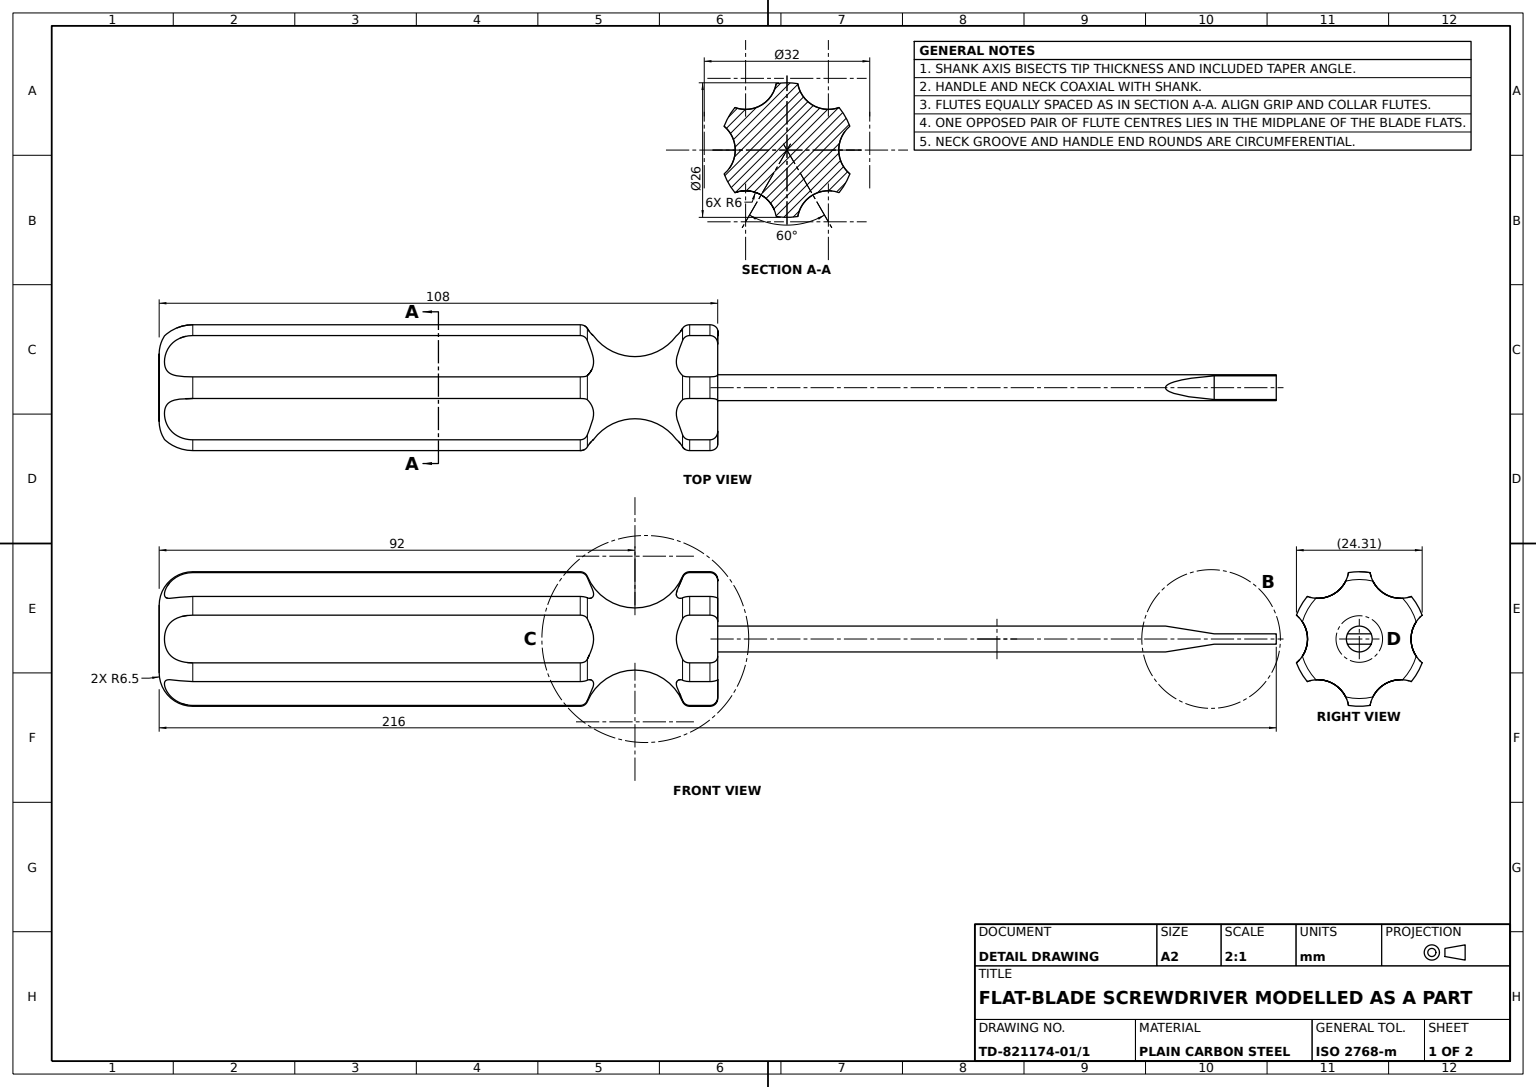
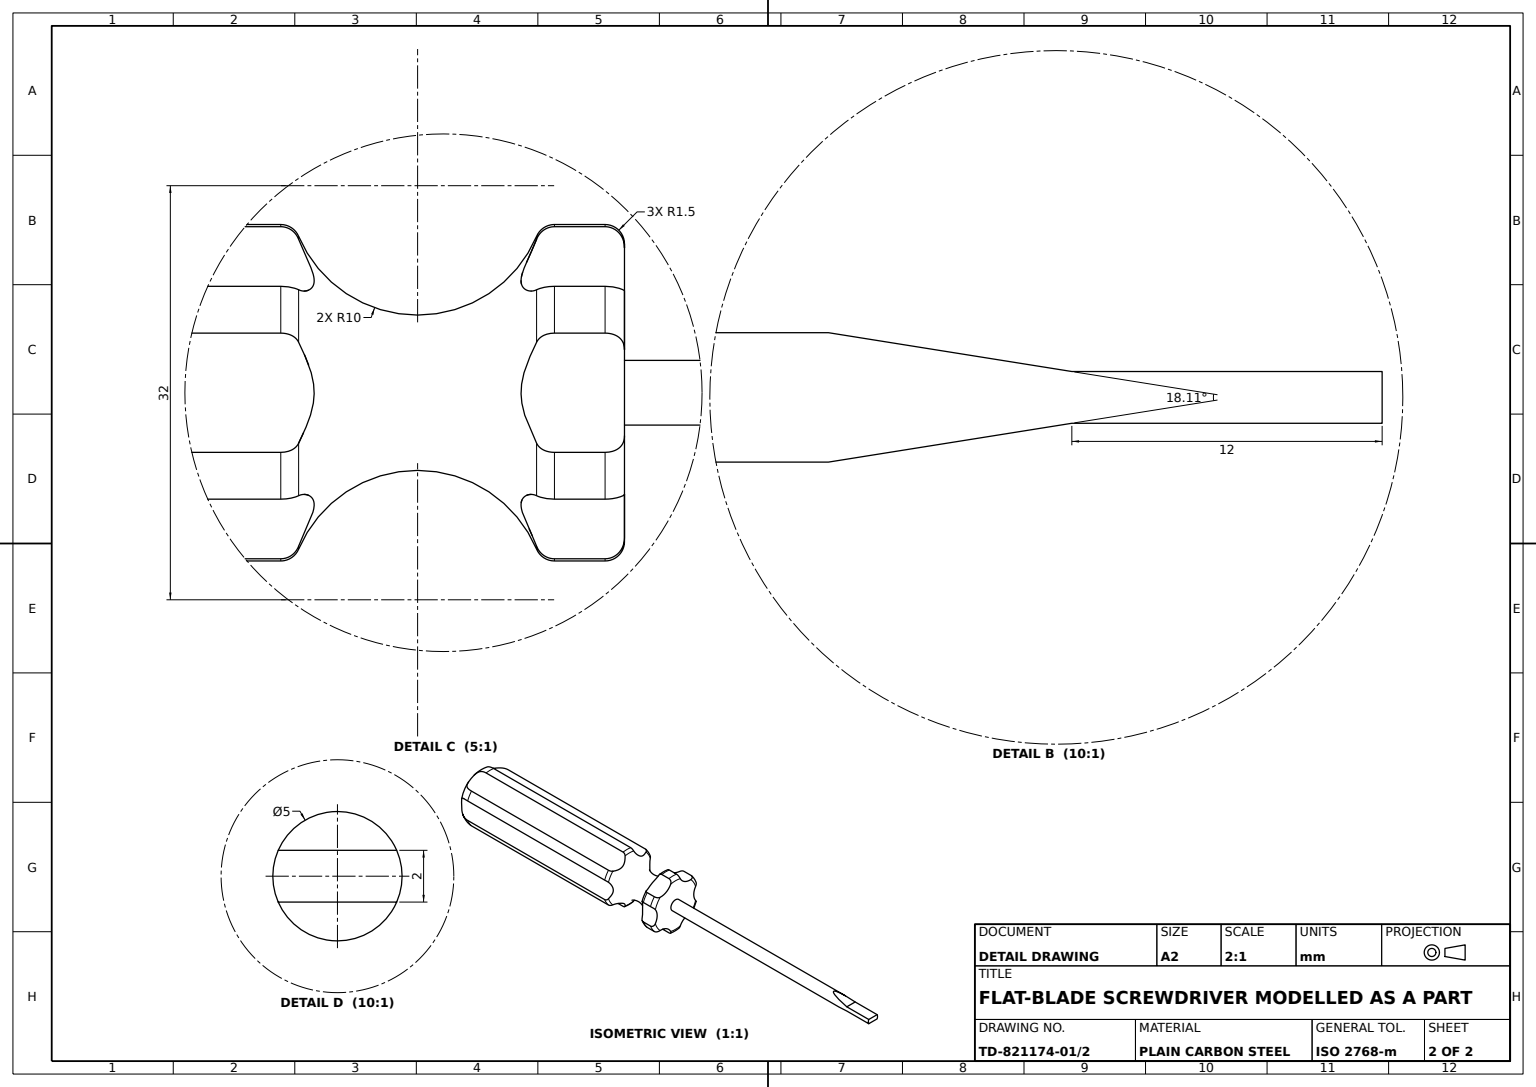
SolidWorks part; units mm, degrees
material "Plain Carbon Steel"
ref_plane "Front Plane" through (0, 0, 0) normal (0, 0, 1) x (1, 0, 0)
ref_plane "Top Plane" through (0, 0, 0) normal (0, 1, 0) x (1, 0, 0)
ref_plane "Right Plane" through (0, 0, 0) normal (1, 0, 0) x (0, 0, -1)
sketch "Handle Profile Sketch" plane through (0, 0, 0) normal (1, 0, 0) x (0, 0, -1)
  line L0 (0, 0) -> (0, 13)
  line L2 (108, 11.5) -> (108, 0)
  line L3 (108, 0) -> (0, 0)
  line L4 (106.5, 13) -> (101.5, 13)
  line L6 (0, 13) -> (101.5, 13)
  arc A2 (106.5, 13) -> (108, 11.5) centre (106.5, 11.5) cw
  point P4 (91.5, 16)
  point P12 (108, 13)
  dimension "D5" = 91.5
  dimension "D7" = 16
  dimension "D4" = 1.5
  dimension "D1" = 108
  dimension "D2" = 13
  dimension "D3" = 6.5
  dimension "D6" = 13
revolve "Handle Body Revolve" add sketch "Handle Profile Sketch" angle 360 about L3
sketch "Flute Lobe Profile Sketch" plane through (0, 0, -108) normal (0, 0, -1) x (-1, 0, 0)
  arc A0 (-4.6071, 12.1562) -> (4.6071, 12.1562) centre (0, 16) ccw
  arc A1 (8.2241, 10.068) -> (12.8312, 2.0882) centre (13.8564, 8) ccw
  arc A2 (12.8312, -2.0882) -> (8.2241, -10.068) centre (13.8564, -8) ccw
  arc A3 (4.6071, -12.1563) -> (-4.6071, -12.1562) centre (0, -16) ccw
  arc A4 (-8.2241, -10.068) -> (-12.8312, -2.0882) centre (-13.8564, -8) ccw
  arc A5 (-12.8312, 2.0882) -> (-8.2241, 10.068) centre (-13.8564, 8) ccw
  circle A6 centre (0, 0) radius 13 construction
  arc A7 (-12.8312, -2.0882) -> (-8.2241, -10.068) centre (0, 0) ccw
  arc A8 (12.8312, 2.0882) -> (8.2241, 10.068) centre (0, 0) ccw
  arc A9 (4.6071, 12.1562) -> (-4.6071, 12.1562) centre (0, 0) ccw
  arc A10 (-8.2241, 10.068) -> (-12.8312, 2.0882) centre (0, 0) ccw
  arc A11 (-4.6071, -12.1562) -> (4.6071, -12.1563) centre (0, 0) ccw
  arc A12 (8.2241, -10.068) -> (12.8312, -2.0882) centre (0, 0) ccw
  point P15 (0, 0)
  dimension "D2" = 12
  dimension "D1" = 16
  dimension "D3" = 6
fillet "Handle End Fillet R6.5" radius 6.5 1 edges at (-13, 0, 0)
extrude "Collar Flute Cut 8.6" cut sketch "Flute Lobe Profile Sketch" against normal blind 8.6
sketch "Neck Groove Sketch" plane through (0, 0, 0) normal (1, 0, 0) x (0, 0, -1)
  line L0 (0, 0) -> (142.1101, 0) construction
  circle A0 centre (92, 16) radius 10
  dimension "D2" = 20
  dimension "D1" = 16
  dimension "D3" = 92
revolve "Neck Groove Cut" cut sketch "Neck Groove Sketch" angle 360 about L0
sketch "Blade Shaft Profile Sketch" plane through (0, 0, 0) normal (1, 0, 0) x (0, 0, -1)
  line L0 (108, 2.6215) -> (108, 8.3864) construction
  line L1 (56, 2.5) -> (216, 2.5)
  line L2 (56, 2.5) -> (56, 0)
  line L4 (216, 2.5) -> (216, 0)
  line L5 (56, 0) -> (216, 0)
  dimension "D1" = 160
  dimension "D2" = 52
  dimension "D3" = 2.5
revolve "Blade Shaft Ø5 Revolve" add sketch "Blade Shaft Profile Sketch" angle 360 about L5
fillet "Groove Edge Fillet R1.5 A" radius 1.5 1 edges at (-13, 0, -82.4606)
fillet "Groove Edge Fillet R1.5 B" radius 1.5 2 edges at (13, 0, -101.5394) (6.5, -11.2583, -101.5394)
fillet "Groove Edge Fillet R1.5 C" radius 1.5 4 edges at (6.5, 11.2583, -101.5394) (-6.5, 11.2583, -101.5394) (-13, 0, -101.5394) (-6.5, -11.2583, -101.5394)
ref_plane "Handle Flute Sketch Plane" through (0, 0, -54) normal (0, 0, 1) x (1, 0, 0)
sketch "Handle Flute Sketch" plane through (0, 0, -54) normal (0, 0, 1) x (1, 0, 0)
  arc A2 (8.2241, 10.068) -> (12.8312, 2.0882) centre (13.8564, 8) ccw
  arc A3 (12.8312, 2.0882) -> (8.2241, 10.068) centre (0, 0) ccw
  arc A4 (8.2241, 10.068) -> (12.8312, 2.0882) centre (13.8564, 8) ccw
  arc A5 (12.8312, 2.0882) -> (8.2241, 10.068) centre (0, 0) ccw
  arc A6 (12.8312, -2.0882) -> (8.2241, -10.068) centre (13.8564, -8) ccw
  arc A7 (8.2241, -10.068) -> (12.8312, -2.0882) centre (0, 0) ccw
  arc A8 (12.8312, -2.0882) -> (8.2241, -10.068) centre (13.8564, -8) ccw
  arc A9 (8.2241, -10.068) -> (12.8312, -2.0882) centre (0, 0) ccw
  arc A10 (4.6071, -12.1562) -> (-4.6071, -12.1563) centre (0, -16) ccw
  arc A11 (-4.6071, -12.1563) -> (4.6071, -12.1562) centre (0, 0) ccw
  arc A12 (4.6071, -12.1562) -> (-4.6071, -12.1563) centre (0, -16) ccw
  arc A13 (-4.6071, -12.1563) -> (4.6071, -12.1562) centre (0, 0) ccw
  arc A14 (-8.2241, -10.068) -> (-12.8312, -2.0882) centre (-13.8564, -8) ccw
  arc A15 (-12.8312, -2.0882) -> (-8.2241, -10.068) centre (0, 0) ccw
  arc A16 (-8.2241, -10.068) -> (-12.8312, -2.0882) centre (-13.8564, -8) ccw
  arc A17 (-12.8312, -2.0882) -> (-8.2241, -10.068) centre (0, 0) ccw
  arc A18 (-12.8312, 2.0882) -> (-8.2241, 10.068) centre (-13.8564, 8) ccw
  arc A19 (-8.2241, 10.068) -> (-12.8312, 2.0882) centre (0, 0) ccw
  arc A20 (-12.8312, 2.0882) -> (-8.2241, 10.068) centre (-13.8564, 8) ccw
  arc A21 (-8.2241, 10.068) -> (-12.8312, 2.0882) centre (0, 0) ccw
  arc A22 (-4.6071, 12.1563) -> (4.6071, 12.1562) centre (0, 16) ccw
  arc A23 (4.6071, 12.1562) -> (-4.6071, 12.1563) centre (0, 0) ccw
  arc A24 (-4.6071, 12.1563) -> (4.6071, 12.1562) centre (0, 16) ccw
  arc A25 (4.6071, 12.1562) -> (-4.6071, 12.1563) centre (0, 0) ccw
  dimension "D1" = 0
  dimension "D2" = 0
  dimension "D3" = 0
  dimension "D4" = 0
  dimension "D5" = 0
  dimension "D6" = 0
extrude "Handle Flutes Cut" cut sketch "Handle Flute Sketch" against normal through all both and the other way through all
sketch "Blade Tip Flat Sketch" plane through (0, 0, 0) normal (0, 1, 0) x (1, 0, 0)
  line L1 (2.5, 216) -> (-2.5, 216) construction
  line L2 (-1, 216) -> (-1, 204)
  line L3 (-1, 204) -> (-2.5, 194.5881)
  line L4 (0, 216) -> (0, 173.1763) construction
  line L5 (-1, 216) -> (-2.5, 216)
  line L6 (-2.5, 216) -> (-2.5, 194.5881)
  dimension "D1" = 12
  dimension "D2" = 1
  dimension "D3" = 2.5
  dimension "D4" = 21.4119
extrude "Blade Tip Flat Cut" cut sketch "Blade Tip Flat Sketch" against normal through all both and the other way through all
mirror "Blade Tip Flat Mirror" about plane through (0, 0, 0) normal (1, 0, 0) of "Blade Tip Flat Cut"
